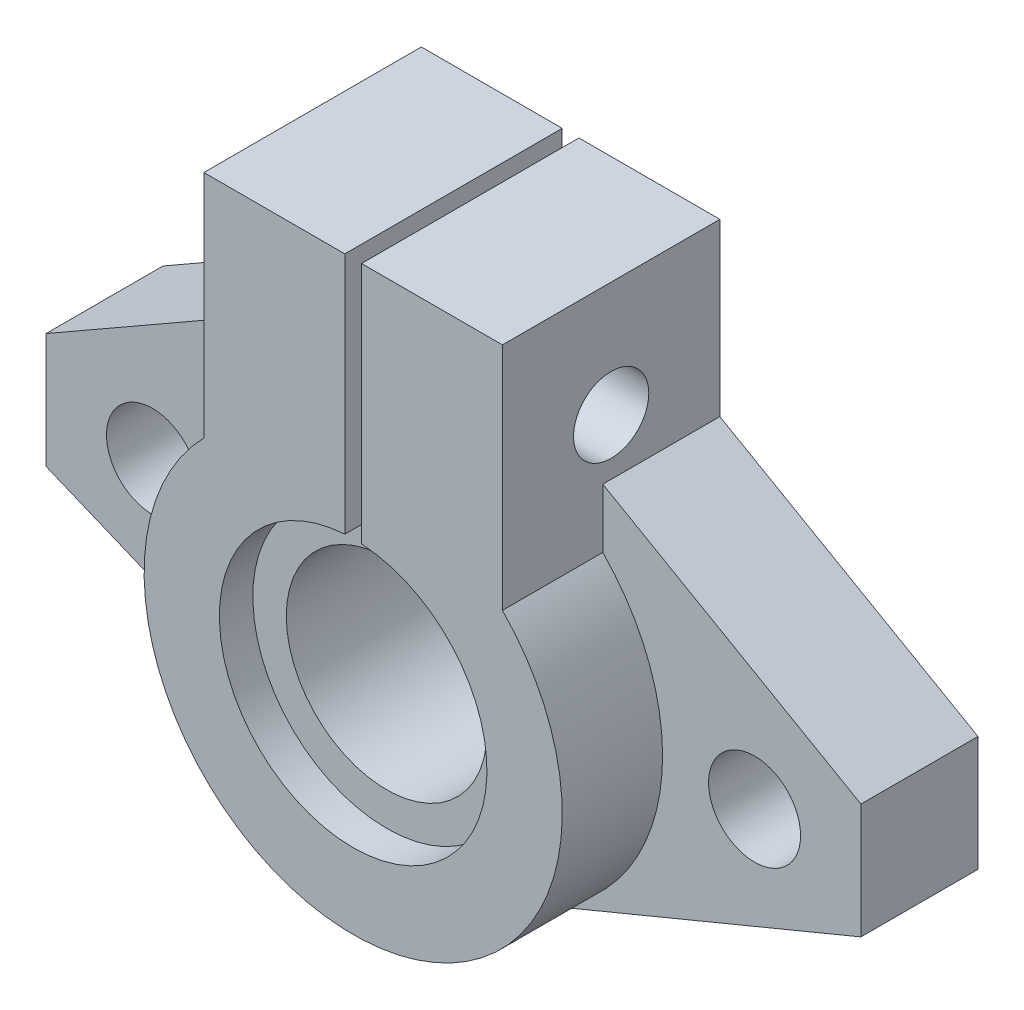
ISO-10303-21;
HEADER;
FILE_DESCRIPTION(('STEP AP214'),'2;1');
FILE_NAME('part.step','',(''),(''),'','','');
FILE_SCHEMA(('AUTOMOTIVE_DESIGN { 1 0 10303 214 1 1 1 1 }'));
ENDSEC;
DATA;
#1=APPLICATION_CONTEXT('core data for automotive mechanical design processes');
#2=APPLICATION_PROTOCOL_DEFINITION('international standard','automotive_design',2000,#1);
#3=PRODUCT_CONTEXT('',#1,'mechanical');
#4=PRODUCT('Part','Part','',(#3));
#5=PRODUCT_RELATED_PRODUCT_CATEGORY('part','',(#4));
#6=PRODUCT_DEFINITION_FORMATION('','',#4);
#7=PRODUCT_DEFINITION_CONTEXT('part definition',#1,'design');
#8=PRODUCT_DEFINITION('design','',#6,#7);
#9=PRODUCT_DEFINITION_SHAPE('','',#8);
#10=(LENGTH_UNIT() NAMED_UNIT(*) SI_UNIT(.MILLI.,.METRE.));
#11=(NAMED_UNIT(*) PLANE_ANGLE_UNIT() SI_UNIT($,.RADIAN.));
#12=(NAMED_UNIT(*) SI_UNIT($,.STERADIAN.) SOLID_ANGLE_UNIT());
#13=UNCERTAINTY_MEASURE_WITH_UNIT(LENGTH_MEASURE(1.E-05),#10,'distance_accuracy_value','');
#14=(GEOMETRIC_REPRESENTATION_CONTEXT(3) GLOBAL_UNCERTAINTY_ASSIGNED_CONTEXT((#13)) GLOBAL_UNIT_ASSIGNED_CONTEXT((#10,
#11,#12)) REPRESENTATION_CONTEXT('',''));
#15=CARTESIAN_POINT('',(0.,0.,0.));
#16=DIRECTION('',(0.,0.,1.));
#17=DIRECTION('',(1.,0.,0.));
#18=AXIS2_PLACEMENT_3D('',#15,#16,#17);
#19=CARTESIAN_POINT('',(-8.925,22.5,13.));
#20=DIRECTION('',(0.,-1.,0.));
#21=DIRECTION('',(0.,0.,-1.));
#22=AXIS2_PLACEMENT_3D('',#19,#20,#21);
#23=PLANE('',#22);
#24=DIRECTION('',(-1.,0.,0.));
#25=VECTOR('',#24,1.);
#26=CARTESIAN_POINT('',(-8.925,22.5,0.));
#27=LINE('',#26,#25);
#28=CARTESIAN_POINT('',(8.925,22.5,0.));
#29=VERTEX_POINT('',#28);
#30=CARTESIAN_POINT('',(0.5,22.5,0.));
#31=VERTEX_POINT('',#30);
#32=EDGE_CURVE('E194',#29,#31,#27,.T.);
#33=ORIENTED_EDGE('',*,*,#32,.T.);
#34=DIRECTION('',(0.,0.,1.));
#35=VECTOR('',#34,1.);
#36=CARTESIAN_POINT('',(0.5,22.5,0.));
#37=LINE('',#36,#35);
#38=CARTESIAN_POINT('',(0.5,22.5,13.));
#39=VERTEX_POINT('',#38);
#40=EDGE_CURVE('E416',#31,#39,#37,.T.);
#41=ORIENTED_EDGE('',*,*,#40,.T.);
#42=DIRECTION('',(-1.,0.,0.));
#43=VECTOR('',#42,1.);
#44=CARTESIAN_POINT('',(-8.925,22.5,13.));
#45=LINE('',#44,#43);
#46=CARTESIAN_POINT('',(8.925,22.5,13.));
#47=VERTEX_POINT('',#46);
#48=EDGE_CURVE('E201',#47,#39,#45,.T.);
#49=ORIENTED_EDGE('',*,*,#48,.F.);
#50=DIRECTION('',(0.,0.,-1.));
#51=VECTOR('',#50,1.);
#52=CARTESIAN_POINT('',(8.925,22.5,13.));
#53=LINE('',#52,#51);
#54=EDGE_CURVE('E205',#47,#29,#53,.T.);
#55=ORIENTED_EDGE('',*,*,#54,.T.);
#56=EDGE_LOOP('',(#33,#41,#49,#55));
#57=FACE_BOUND('',#56,.T.);
#58=ADVANCED_FACE('F43',(#57),#23,.F.);
#59=CARTESIAN_POINT('',(0.,0.,13.));
#60=DIRECTION('',(0.,0.,-1.));
#61=DIRECTION('',(-1.,0.,0.));
#62=AXIS2_PLACEMENT_3D('',#59,#60,#61);
#63=CYLINDRICAL_SURFACE('',#62,12.5);
#64=DIRECTION('',(0.,0.,-1.));
#65=VECTOR('',#64,1.);
#66=CARTESIAN_POINT('',(4.78354290456363,-11.5484941563911,7.));
#67=LINE('',#66,#65);
#68=CARTESIAN_POINT('',(4.78354290456363,-11.5484941563911,7.));
#69=VERTEX_POINT('',#68);
#70=CARTESIAN_POINT('',(4.78354290456363,-11.5484941563911,0.));
#71=VERTEX_POINT('',#70);
#72=EDGE_CURVE('E261',#69,#71,#67,.T.);
#73=ORIENTED_EDGE('',*,*,#72,.F.);
#74=CARTESIAN_POINT('',(0.,0.,7.));
#75=DIRECTION('',(0.,0.,1.));
#76=DIRECTION('',(1.,0.,0.));
#77=AXIS2_PLACEMENT_3D('',#74,#75,#76);
#78=CIRCLE('',#77,12.5);
#79=CARTESIAN_POINT('',(8.925,8.75182123903362,7.));
#80=VERTEX_POINT('',#79);
#81=EDGE_CURVE('E377',#69,#80,#78,.T.);
#82=ORIENTED_EDGE('',*,*,#81,.T.);
#83=DIRECTION('',(0.,0.,-1.));
#84=VECTOR('',#83,1.);
#85=CARTESIAN_POINT('',(8.925,8.75182123903362,13.));
#86=LINE('',#85,#84);
#87=CARTESIAN_POINT('',(8.925,8.75182123903362,13.));
#88=VERTEX_POINT('',#87);
#89=EDGE_CURVE('E206',#88,#80,#86,.T.);
#90=ORIENTED_EDGE('',*,*,#89,.F.);
#91=CARTESIAN_POINT('',(0.,0.,13.));
#92=DIRECTION('',(0.,0.,1.));
#93=DIRECTION('',(1.,0.,0.));
#94=AXIS2_PLACEMENT_3D('',#91,#92,#93);
#95=CIRCLE('',#94,12.5);
#96=CARTESIAN_POINT('',(-8.925,8.75182123903362,13.));
#97=VERTEX_POINT('',#96);
#98=EDGE_CURVE('E213',#97,#88,#95,.T.);
#99=ORIENTED_EDGE('',*,*,#98,.F.);
#100=DIRECTION('',(0.,0.,-1.));
#101=VECTOR('',#100,1.);
#102=CARTESIAN_POINT('',(-8.925,8.75182123903362,13.));
#103=LINE('',#102,#101);
#104=CARTESIAN_POINT('',(-8.925,8.75182123903362,7.));
#105=VERTEX_POINT('',#104);
#106=EDGE_CURVE('E207',#97,#105,#103,.T.);
#107=ORIENTED_EDGE('',*,*,#106,.T.);
#108=CARTESIAN_POINT('',(0.,0.,7.));
#109=DIRECTION('',(0.,0.,1.));
#110=DIRECTION('',(1.,0.,0.));
#111=AXIS2_PLACEMENT_3D('',#108,#109,#110);
#112=CIRCLE('',#111,12.5);
#113=CARTESIAN_POINT('',(-4.78354290456363,-11.5484941563911,7.));
#114=VERTEX_POINT('',#113);
#115=EDGE_CURVE('E277',#105,#114,#112,.T.);
#116=ORIENTED_EDGE('',*,*,#115,.T.);
#117=DIRECTION('',(0.,0.,-1.));
#118=VECTOR('',#117,1.);
#119=CARTESIAN_POINT('',(-4.78354290456363,-11.5484941563911,7.));
#120=LINE('',#119,#118);
#121=CARTESIAN_POINT('',(-4.78354290456363,-11.5484941563911,0.));
#122=VERTEX_POINT('',#121);
#123=EDGE_CURVE('E280',#114,#122,#120,.T.);
#124=ORIENTED_EDGE('',*,*,#123,.T.);
#125=CARTESIAN_POINT('',(0.,0.,0.));
#126=DIRECTION('',(0.,0.,1.));
#127=DIRECTION('',(1.,0.,0.));
#128=AXIS2_PLACEMENT_3D('',#125,#126,#127);
#129=CIRCLE('',#128,12.5);
#130=EDGE_CURVE('E215',#122,#71,#129,.T.);
#131=ORIENTED_EDGE('',*,*,#130,.T.);
#132=EDGE_LOOP('',(#73,#82,#90,#99,#107,#116,#124,#131));
#133=FACE_BOUND('',#132,.T.);
#134=ADVANCED_FACE('F44',(#133),#63,.T.);
#135=CARTESIAN_POINT('',(8.925,22.5,13.));
#136=DIRECTION('',(-1.,0.,0.));
#137=DIRECTION('',(0.,0.,1.));
#138=AXIS2_PLACEMENT_3D('',#135,#136,#137);
#139=PLANE('',#138);
#140=CARTESIAN_POINT('',(8.925,15.6259106195168,6.5));
#141=DIRECTION('',(1.,0.,0.));
#142=DIRECTION('',(0.,0.,-1.));
#143=AXIS2_PLACEMENT_3D('',#140,#141,#142);
#144=CIRCLE('',#143,2.25);
#145=CARTESIAN_POINT('',(8.925,15.6259106195168,4.25));
#146=VERTEX_POINT('',#145);
#147=EDGE_CURVE('E436',#146,#146,#144,.T.);
#148=ORIENTED_EDGE('',*,*,#147,.F.);
#149=EDGE_LOOP('',(#148));
#150=FACE_BOUND('',#149,.T.);
#151=DIRECTION('',(0.,0.,-1.));
#152=VECTOR('',#151,1.);
#153=CARTESIAN_POINT('',(8.925,12.2859520739162,7.));
#154=LINE('',#153,#152);
#155=CARTESIAN_POINT('',(8.925,12.2859520739162,7.));
#156=VERTEX_POINT('',#155);
#157=CARTESIAN_POINT('',(8.925,12.2859520739162,0.));
#158=VERTEX_POINT('',#157);
#159=EDGE_CURVE('E402',#156,#158,#154,.T.);
#160=ORIENTED_EDGE('',*,*,#159,.T.);
#161=DIRECTION('',(0.,1.,0.));
#162=VECTOR('',#161,1.);
#163=CARTESIAN_POINT('',(8.925,22.5,0.));
#164=LINE('',#163,#162);
#165=EDGE_CURVE('E195',#158,#29,#164,.T.);
#166=ORIENTED_EDGE('',*,*,#165,.T.);
#167=ORIENTED_EDGE('',*,*,#54,.F.);
#168=DIRECTION('',(0.,1.,0.));
#169=VECTOR('',#168,1.);
#170=CARTESIAN_POINT('',(8.925,22.5,13.));
#171=LINE('',#170,#169);
#172=EDGE_CURVE('E243',#88,#47,#171,.T.);
#173=ORIENTED_EDGE('',*,*,#172,.F.);
#174=ORIENTED_EDGE('',*,*,#89,.T.);
#175=DIRECTION('',(0.,-1.,0.));
#176=VECTOR('',#175,1.);
#177=CARTESIAN_POINT('',(8.925,0.,7.));
#178=LINE('',#177,#176);
#179=EDGE_CURVE('E384',#156,#80,#178,.T.);
#180=ORIENTED_EDGE('',*,*,#179,.F.);
#181=EDGE_LOOP('',(#160,#166,#167,#173,#174,#180));
#182=FACE_BOUND('',#181,.T.);
#183=ADVANCED_FACE('F324',(#150,#182),#139,.F.);
#184=CARTESIAN_POINT('',(0.,0.,0.));
#185=DIRECTION('',(0.,0.,1.));
#186=DIRECTION('',(1.,0.,0.));
#187=AXIS2_PLACEMENT_3D('',#184,#185,#186);
#188=CYLINDRICAL_SURFACE('',#187,6.);
#189=CARTESIAN_POINT('',(0.,0.,11.));
#190=DIRECTION('',(0.,0.,1.));
#191=DIRECTION('',(1.,0.,0.));
#192=AXIS2_PLACEMENT_3D('',#189,#190,#191);
#193=CIRCLE('',#192,6.);
#194=CARTESIAN_POINT('',(0.5,5.9791303715507,11.));
#195=VERTEX_POINT('',#194);
#196=CARTESIAN_POINT('',(-0.5,5.9791303715507,11.));
#197=VERTEX_POINT('',#196);
#198=EDGE_CURVE('E220',#195,#197,#193,.F.);
#199=ORIENTED_EDGE('',*,*,#198,.F.);
#200=DIRECTION('',(0.,0.,1.));
#201=VECTOR('',#200,1.);
#202=CARTESIAN_POINT('',(0.5,5.9791303715507,0.));
#203=LINE('',#202,#201);
#204=CARTESIAN_POINT('',(0.5,5.9791303715507,0.));
#205=VERTEX_POINT('',#204);
#206=EDGE_CURVE('E423',#205,#195,#203,.T.);
#207=ORIENTED_EDGE('',*,*,#206,.F.);
#208=CARTESIAN_POINT('',(0.,0.,0.));
#209=DIRECTION('',(0.,0.,1.));
#210=DIRECTION('',(1.,0.,0.));
#211=AXIS2_PLACEMENT_3D('',#208,#209,#210);
#212=CIRCLE('',#211,6.);
#213=CARTESIAN_POINT('',(-0.5,5.9791303715507,0.));
#214=VERTEX_POINT('',#213);
#215=EDGE_CURVE('E219',#214,#205,#212,.T.);
#216=ORIENTED_EDGE('',*,*,#215,.F.);
#217=DIRECTION('',(0.,0.,1.));
#218=VECTOR('',#217,1.);
#219=CARTESIAN_POINT('',(-0.5,5.9791303715507,0.));
#220=LINE('',#219,#218);
#221=EDGE_CURVE('E171',#214,#197,#220,.T.);
#222=ORIENTED_EDGE('',*,*,#221,.T.);
#223=EDGE_LOOP('',(#199,#207,#216,#222));
#224=FACE_BOUND('',#223,.T.);
#225=ADVANCED_FACE('F350',(#224),#188,.F.);
#226=CARTESIAN_POINT('',(0.,0.,13.));
#227=DIRECTION('',(0.,0.,1.));
#228=DIRECTION('',(1.,0.,0.));
#229=AXIS2_PLACEMENT_3D('',#226,#227,#228);
#230=PLANE('',#229);
#231=DIRECTION('',(0.,1.,0.));
#232=VECTOR('',#231,1.);
#233=CARTESIAN_POINT('',(0.5,5.9791303715507,13.));
#234=LINE('',#233,#232);
#235=CARTESIAN_POINT('',(0.5,7.98435971133565,13.));
#236=VERTEX_POINT('',#235);
#237=EDGE_CURVE('E179',#236,#39,#234,.T.);
#238=ORIENTED_EDGE('',*,*,#237,.F.);
#239=CARTESIAN_POINT('',(0.,0.,13.));
#240=DIRECTION('',(0.,0.,1.));
#241=DIRECTION('',(1.,0.,0.));
#242=AXIS2_PLACEMENT_3D('',#239,#240,#241);
#243=CIRCLE('',#242,8.);
#244=CARTESIAN_POINT('',(-0.5,7.98435971133565,13.));
#245=VERTEX_POINT('',#244);
#246=EDGE_CURVE('E227',#245,#236,#243,.T.);
#247=ORIENTED_EDGE('',*,*,#246,.F.);
#248=DIRECTION('',(0.,-1.,0.));
#249=VECTOR('',#248,1.);
#250=CARTESIAN_POINT('',(-0.5,5.9791303715507,13.));
#251=LINE('',#250,#249);
#252=CARTESIAN_POINT('',(-0.5,22.5,13.));
#253=VERTEX_POINT('',#252);
#254=EDGE_CURVE('E56',#253,#245,#251,.T.);
#255=ORIENTED_EDGE('',*,*,#254,.F.);
#256=CARTESIAN_POINT('',(-8.925,22.5,13.));
#257=VERTEX_POINT('',#256);
#258=EDGE_CURVE('E183',#253,#257,#45,.T.);
#259=ORIENTED_EDGE('',*,*,#258,.T.);
#260=DIRECTION('',(0.,-1.,0.));
#261=VECTOR('',#260,1.);
#262=CARTESIAN_POINT('',(-8.925,22.5,13.));
#263=LINE('',#262,#261);
#264=EDGE_CURVE('E198',#257,#97,#263,.T.);
#265=ORIENTED_EDGE('',*,*,#264,.T.);
#266=ORIENTED_EDGE('',*,*,#98,.T.);
#267=ORIENTED_EDGE('',*,*,#172,.T.);
#268=ORIENTED_EDGE('',*,*,#48,.T.);
#269=EDGE_LOOP('',(#238,#247,#255,#259,#265,#266,#267,#268));
#270=FACE_BOUND('',#269,.T.);
#271=ADVANCED_FACE('F234',(#270),#230,.T.);
#272=CARTESIAN_POINT('',(0.,0.,0.));
#273=DIRECTION('',(0.,0.,1.));
#274=DIRECTION('',(1.,0.,0.));
#275=AXIS2_PLACEMENT_3D('',#272,#273,#274);
#276=PLANE('',#275);
#277=ORIENTED_EDGE('',*,*,#215,.T.);
#278=DIRECTION('',(0.,1.,0.));
#279=VECTOR('',#278,1.);
#280=CARTESIAN_POINT('',(0.5,5.9791303715507,0.));
#281=LINE('',#280,#279);
#282=EDGE_CURVE('E177',#205,#31,#281,.T.);
#283=ORIENTED_EDGE('',*,*,#282,.T.);
#284=ORIENTED_EDGE('',*,*,#32,.F.);
#285=ORIENTED_EDGE('',*,*,#165,.F.);
#286=DIRECTION('',(-0.867602640598347,0.497258140231787,0.));
#287=VECTOR('',#286,1.);
#288=CARTESIAN_POINT('',(7.5072818557886,13.0985036439266,0.));
#289=LINE('',#288,#287);
#290=CARTESIAN_POINT('',(24.3591794673459,3.44,0.));
#291=VERTEX_POINT('',#290);
#292=EDGE_CURVE('E386',#291,#158,#289,.T.);
#293=ORIENTED_EDGE('',*,*,#292,.F.);
#294=DIRECTION('',(0.,-1.,0.));
#295=VECTOR('',#294,1.);
#296=CARTESIAN_POINT('',(24.3591794673459,0.,0.));
#297=LINE('',#296,#295);
#298=CARTESIAN_POINT('',(24.3591794673459,-3.44,0.));
#299=VERTEX_POINT('',#298);
#300=EDGE_CURVE('E401',#291,#299,#297,.T.);
#301=ORIENTED_EDGE('',*,*,#300,.T.);
#302=DIRECTION('',(0.923879532511287,0.38268343236509,0.));
#303=VECTOR('',#302,1.);
#304=CARTESIAN_POINT('',(4.78354290456363,-11.5484941563911,0.));
#305=LINE('',#304,#303);
#306=EDGE_CURVE('E367',#71,#299,#305,.T.);
#307=ORIENTED_EDGE('',*,*,#306,.F.);
#308=ORIENTED_EDGE('',*,*,#130,.F.);
#309=DIRECTION('',(-0.923879532511287,0.38268343236509,0.));
#310=VECTOR('',#309,1.);
#311=CARTESIAN_POINT('',(-4.78354290456363,-11.5484941563911,0.));
#312=LINE('',#311,#310);
#313=CARTESIAN_POINT('',(-24.3661310458058,-3.43712056192201,0.));
#314=VERTEX_POINT('',#313);
#315=EDGE_CURVE('E263',#122,#314,#312,.T.);
#316=ORIENTED_EDGE('',*,*,#315,.T.);
#317=DIRECTION('',(0.,-1.,0.));
#318=VECTOR('',#317,1.);
#319=CARTESIAN_POINT('',(-24.3661310458058,0.,0.));
#320=LINE('',#319,#318);
#321=CARTESIAN_POINT('',(-24.3661310458058,3.44,0.));
#322=VERTEX_POINT('',#321);
#323=EDGE_CURVE('E257',#322,#314,#320,.T.);
#324=ORIENTED_EDGE('',*,*,#323,.F.);
#325=DIRECTION('',(0.86769921537807,0.497089601211171,0.));
#326=VECTOR('',#325,1.);
#327=CARTESIAN_POINT('',(-7.50457943844383,13.0996860015059,0.));
#328=LINE('',#327,#326);
#329=CARTESIAN_POINT('',(-8.925,12.2859520739162,0.));
#330=VERTEX_POINT('',#329);
#331=EDGE_CURVE('E255',#322,#330,#328,.T.);
#332=ORIENTED_EDGE('',*,*,#331,.T.);
#333=DIRECTION('',(0.,-1.,0.));
#334=VECTOR('',#333,1.);
#335=CARTESIAN_POINT('',(-8.925,22.5,0.));
#336=LINE('',#335,#334);
#337=CARTESIAN_POINT('',(-8.925,22.5,0.));
#338=VERTEX_POINT('',#337);
#339=EDGE_CURVE('E192',#338,#330,#336,.T.);
#340=ORIENTED_EDGE('',*,*,#339,.F.);
#341=CARTESIAN_POINT('',(-0.5,22.5,0.));
#342=VERTEX_POINT('',#341);
#343=EDGE_CURVE('E181',#342,#338,#27,.T.);
#344=ORIENTED_EDGE('',*,*,#343,.F.);
#345=DIRECTION('',(0.,-1.,0.));
#346=VECTOR('',#345,1.);
#347=CARTESIAN_POINT('',(-0.5,5.9791303715507,0.));
#348=LINE('',#347,#346);
#349=EDGE_CURVE('E167',#342,#214,#348,.T.);
#350=ORIENTED_EDGE('',*,*,#349,.T.);
#351=EDGE_LOOP('',(#277,#283,#284,#285,#293,#301,#307,#308,#316,#324,#332,#340,#344,#350));
#352=FACE_BOUND('',#351,.T.);
#353=CARTESIAN_POINT('',(-18.,0.,0.));
#354=DIRECTION('',(0.,0.,1.));
#355=DIRECTION('',(1.,0.,0.));
#356=AXIS2_PLACEMENT_3D('',#353,#354,#355);
#357=CIRCLE('',#356,2.75);
#358=CARTESIAN_POINT('',(-15.25,0.,0.));
#359=VERTEX_POINT('',#358);
#360=EDGE_CURVE('E272',#359,#359,#357,.T.);
#361=ORIENTED_EDGE('',*,*,#360,.T.);
#362=EDGE_LOOP('',(#361));
#363=FACE_BOUND('',#362,.T.);
#364=CARTESIAN_POINT('',(18.,0.,0.));
#365=DIRECTION('',(0.,0.,1.));
#366=DIRECTION('',(1.,0.,0.));
#367=AXIS2_PLACEMENT_3D('',#364,#365,#366);
#368=CIRCLE('',#367,2.75);
#369=CARTESIAN_POINT('',(20.75,0.,0.));
#370=VERTEX_POINT('',#369);
#371=EDGE_CURVE('E387',#370,#370,#368,.T.);
#372=ORIENTED_EDGE('',*,*,#371,.T.);
#373=EDGE_LOOP('',(#372));
#374=FACE_BOUND('',#373,.T.);
#375=ADVANCED_FACE('F189',(#352,#363,#374),#276,.F.);
#376=CARTESIAN_POINT('',(-8.925,22.5,13.));
#377=DIRECTION('',(1.,0.,0.));
#378=DIRECTION('',(0.,0.,-1.));
#379=AXIS2_PLACEMENT_3D('',#376,#377,#378);
#380=PLANE('',#379);
#381=CARTESIAN_POINT('',(-8.925,15.6259106195168,6.5));
#382=DIRECTION('',(1.,0.,0.));
#383=DIRECTION('',(0.,0.,-1.));
#384=AXIS2_PLACEMENT_3D('',#381,#382,#383);
#385=CIRCLE('',#384,2.25);
#386=CARTESIAN_POINT('',(-8.925,15.6259106195168,4.25));
#387=VERTEX_POINT('',#386);
#388=EDGE_CURVE('E429',#387,#387,#385,.T.);
#389=ORIENTED_EDGE('',*,*,#388,.T.);
#390=EDGE_LOOP('',(#389));
#391=FACE_BOUND('',#390,.T.);
#392=ORIENTED_EDGE('',*,*,#339,.T.);
#393=DIRECTION('',(0.,0.,-1.));
#394=VECTOR('',#393,1.);
#395=CARTESIAN_POINT('',(-8.925,12.2859520739162,7.));
#396=LINE('',#395,#394);
#397=CARTESIAN_POINT('',(-8.925,12.2859520739162,7.));
#398=VERTEX_POINT('',#397);
#399=EDGE_CURVE('E231',#398,#330,#396,.T.);
#400=ORIENTED_EDGE('',*,*,#399,.F.);
#401=DIRECTION('',(0.,-1.,0.));
#402=VECTOR('',#401,1.);
#403=CARTESIAN_POINT('',(-8.925,0.,7.));
#404=LINE('',#403,#402);
#405=EDGE_CURVE('E294',#398,#105,#404,.T.);
#406=ORIENTED_EDGE('',*,*,#405,.T.);
#407=ORIENTED_EDGE('',*,*,#106,.F.);
#408=ORIENTED_EDGE('',*,*,#264,.F.);
#409=DIRECTION('',(0.,0.,-1.));
#410=VECTOR('',#409,1.);
#411=CARTESIAN_POINT('',(-8.925,22.5,13.));
#412=LINE('',#411,#410);
#413=EDGE_CURVE('E199',#257,#338,#412,.T.);
#414=ORIENTED_EDGE('',*,*,#413,.T.);
#415=EDGE_LOOP('',(#392,#400,#406,#407,#408,#414));
#416=FACE_BOUND('',#415,.T.);
#417=ADVANCED_FACE('F249',(#391,#416),#380,.F.);
#418=ORIENTED_EDGE('',*,*,#258,.F.);
#419=DIRECTION('',(0.,0.,1.));
#420=VECTOR('',#419,1.);
#421=CARTESIAN_POINT('',(-0.5,22.5,0.));
#422=LINE('',#421,#420);
#423=EDGE_CURVE('E166',#342,#253,#422,.T.);
#424=ORIENTED_EDGE('',*,*,#423,.F.);
#425=ORIENTED_EDGE('',*,*,#343,.T.);
#426=ORIENTED_EDGE('',*,*,#413,.F.);
#427=EDGE_LOOP('',(#418,#424,#425,#426));
#428=FACE_BOUND('',#427,.T.);
#429=ADVANCED_FACE('F182',(#428),#23,.F.);
#430=CARTESIAN_POINT('',(0.,0.,11.));
#431=DIRECTION('',(0.,0.,1.));
#432=DIRECTION('',(1.,0.,0.));
#433=AXIS2_PLACEMENT_3D('',#430,#431,#432);
#434=PLANE('',#433);
#435=DIRECTION('',(0.,1.,0.));
#436=VECTOR('',#435,1.);
#437=CARTESIAN_POINT('',(0.5,0.,11.));
#438=LINE('',#437,#436);
#439=CARTESIAN_POINT('',(0.5,7.98435971133565,11.));
#440=VERTEX_POINT('',#439);
#441=EDGE_CURVE('E69',#195,#440,#438,.T.);
#442=ORIENTED_EDGE('',*,*,#441,.F.);
#443=ORIENTED_EDGE('',*,*,#198,.T.);
#444=DIRECTION('',(0.,-1.,0.));
#445=VECTOR('',#444,1.);
#446=CARTESIAN_POINT('',(-0.5,0.,11.));
#447=LINE('',#446,#445);
#448=CARTESIAN_POINT('',(-0.5,7.98435971133565,11.));
#449=VERTEX_POINT('',#448);
#450=EDGE_CURVE('E419',#449,#197,#447,.T.);
#451=ORIENTED_EDGE('',*,*,#450,.F.);
#452=CARTESIAN_POINT('',(0.,0.,11.));
#453=DIRECTION('',(0.,0.,1.));
#454=DIRECTION('',(1.,0.,0.));
#455=AXIS2_PLACEMENT_3D('',#452,#453,#454);
#456=CIRCLE('',#455,8.);
#457=EDGE_CURVE('E222',#449,#440,#456,.T.);
#458=ORIENTED_EDGE('',*,*,#457,.T.);
#459=EDGE_LOOP('',(#442,#443,#451,#458));
#460=FACE_BOUND('',#459,.T.);
#461=ADVANCED_FACE('F329',(#460),#434,.T.);
#462=CARTESIAN_POINT('',(0.,0.,11.));
#463=DIRECTION('',(0.,0.,1.));
#464=DIRECTION('',(1.,0.,0.));
#465=AXIS2_PLACEMENT_3D('',#462,#463,#464);
#466=CYLINDRICAL_SURFACE('',#465,8.);
#467=ORIENTED_EDGE('',*,*,#246,.T.);
#468=DIRECTION('',(0.,0.,1.));
#469=VECTOR('',#468,1.);
#470=CARTESIAN_POINT('',(0.5,7.98435971133565,11.));
#471=LINE('',#470,#469);
#472=EDGE_CURVE('E11',#236,#440,#471,.F.);
#473=ORIENTED_EDGE('',*,*,#472,.T.);
#474=ORIENTED_EDGE('',*,*,#457,.F.);
#475=DIRECTION('',(0.,0.,1.));
#476=VECTOR('',#475,1.);
#477=CARTESIAN_POINT('',(-0.5,7.98435971133565,11.));
#478=LINE('',#477,#476);
#479=EDGE_CURVE('E55',#449,#245,#478,.T.);
#480=ORIENTED_EDGE('',*,*,#479,.T.);
#481=EDGE_LOOP('',(#467,#473,#474,#480));
#482=FACE_BOUND('',#481,.T.);
#483=ADVANCED_FACE('F226',(#482),#466,.F.);
#484=CARTESIAN_POINT('',(-7.50457943844383,13.0996860015059,7.));
#485=DIRECTION('',(-0.497089601211171,0.86769921537807,0.));
#486=DIRECTION('',(-0.86769921537807,-0.497089601211171,0.));
#487=AXIS2_PLACEMENT_3D('',#484,#485,#486);
#488=PLANE('',#487);
#489=ORIENTED_EDGE('',*,*,#331,.F.);
#490=DIRECTION('',(0.,0.,-1.));
#491=VECTOR('',#490,1.);
#492=CARTESIAN_POINT('',(-24.3661310458058,3.44,7.));
#493=LINE('',#492,#491);
#494=CARTESIAN_POINT('',(-24.3661310458058,3.44,7.));
#495=VERTEX_POINT('',#494);
#496=EDGE_CURVE('E236',#495,#322,#493,.T.);
#497=ORIENTED_EDGE('',*,*,#496,.F.);
#498=DIRECTION('',(0.86769921537807,0.497089601211171,0.));
#499=VECTOR('',#498,1.);
#500=CARTESIAN_POINT('',(-7.50457943844383,13.0996860015059,7.));
#501=LINE('',#500,#499);
#502=EDGE_CURVE('E258',#495,#398,#501,.T.);
#503=ORIENTED_EDGE('',*,*,#502,.T.);
#504=ORIENTED_EDGE('',*,*,#399,.T.);
#505=EDGE_LOOP('',(#489,#497,#503,#504));
#506=FACE_BOUND('',#505,.T.);
#507=ADVANCED_FACE('F251',(#506),#488,.T.);
#508=CARTESIAN_POINT('',(-24.3661310458058,0.,7.));
#509=DIRECTION('',(1.,0.,0.));
#510=DIRECTION('',(0.,0.,-1.));
#511=AXIS2_PLACEMENT_3D('',#508,#509,#510);
#512=PLANE('',#511);
#513=ORIENTED_EDGE('',*,*,#323,.T.);
#514=DIRECTION('',(0.,0.,-1.));
#515=VECTOR('',#514,1.);
#516=CARTESIAN_POINT('',(-24.3661310458058,-3.43712056192201,7.));
#517=LINE('',#516,#515);
#518=CARTESIAN_POINT('',(-24.3661310458058,-3.43712056192201,7.));
#519=VERTEX_POINT('',#518);
#520=EDGE_CURVE('E276',#519,#314,#517,.T.);
#521=ORIENTED_EDGE('',*,*,#520,.F.);
#522=DIRECTION('',(0.,-1.,0.));
#523=VECTOR('',#522,1.);
#524=CARTESIAN_POINT('',(-24.3661310458058,0.,7.));
#525=LINE('',#524,#523);
#526=EDGE_CURVE('E285',#495,#519,#525,.T.);
#527=ORIENTED_EDGE('',*,*,#526,.F.);
#528=ORIENTED_EDGE('',*,*,#496,.T.);
#529=EDGE_LOOP('',(#513,#521,#527,#528));
#530=FACE_BOUND('',#529,.T.);
#531=ADVANCED_FACE('F284',(#530),#512,.F.);
#532=CARTESIAN_POINT('',(-4.78354290456363,-11.5484941563911,7.));
#533=DIRECTION('',(-0.38268343236509,-0.923879532511287,0.));
#534=DIRECTION('',(0.923879532511287,-0.38268343236509,0.));
#535=AXIS2_PLACEMENT_3D('',#532,#533,#534);
#536=PLANE('',#535);
#537=ORIENTED_EDGE('',*,*,#315,.F.);
#538=ORIENTED_EDGE('',*,*,#123,.F.);
#539=DIRECTION('',(-0.923879532511287,0.38268343236509,0.));
#540=VECTOR('',#539,1.);
#541=CARTESIAN_POINT('',(-4.78354290456363,-11.5484941563911,7.));
#542=LINE('',#541,#540);
#543=EDGE_CURVE('E286',#114,#519,#542,.T.);
#544=ORIENTED_EDGE('',*,*,#543,.T.);
#545=ORIENTED_EDGE('',*,*,#520,.T.);
#546=EDGE_LOOP('',(#537,#538,#544,#545));
#547=FACE_BOUND('',#546,.T.);
#548=ADVANCED_FACE('F312',(#547),#536,.T.);
#549=CARTESIAN_POINT('',(-18.,0.,7.));
#550=DIRECTION('',(0.,0.,-1.));
#551=DIRECTION('',(-1.,0.,0.));
#552=AXIS2_PLACEMENT_3D('',#549,#550,#551);
#553=CYLINDRICAL_SURFACE('',#552,2.75);
#554=CARTESIAN_POINT('',(-18.,0.,7.));
#555=DIRECTION('',(0.,0.,1.));
#556=DIRECTION('',(1.,0.,0.));
#557=AXIS2_PLACEMENT_3D('',#554,#555,#556);
#558=CIRCLE('',#557,2.75);
#559=CARTESIAN_POINT('',(-15.25,0.,7.));
#560=VERTEX_POINT('',#559);
#561=EDGE_CURVE('E267',#560,#560,#558,.T.);
#562=ORIENTED_EDGE('',*,*,#561,.T.);
#563=EDGE_LOOP('',(#562));
#564=FACE_BOUND('',#563,.T.);
#565=ORIENTED_EDGE('',*,*,#360,.F.);
#566=EDGE_LOOP('',(#565));
#567=FACE_BOUND('',#566,.T.);
#568=ADVANCED_FACE('F305',(#564,#567),#553,.F.);
#569=CARTESIAN_POINT('',(0.,0.,7.));
#570=DIRECTION('',(0.,0.,1.));
#571=DIRECTION('',(1.,0.,0.));
#572=AXIS2_PLACEMENT_3D('',#569,#570,#571);
#573=PLANE('',#572);
#574=ORIENTED_EDGE('',*,*,#115,.F.);
#575=ORIENTED_EDGE('',*,*,#405,.F.);
#576=ORIENTED_EDGE('',*,*,#502,.F.);
#577=ORIENTED_EDGE('',*,*,#526,.T.);
#578=ORIENTED_EDGE('',*,*,#543,.F.);
#579=EDGE_LOOP('',(#574,#575,#576,#577,#578));
#580=FACE_BOUND('',#579,.T.);
#581=ORIENTED_EDGE('',*,*,#561,.F.);
#582=EDGE_LOOP('',(#581));
#583=FACE_BOUND('',#582,.T.);
#584=ADVANCED_FACE('F295',(#580,#583),#573,.T.);
#585=CARTESIAN_POINT('',(4.78354290456363,-11.5484941563911,7.));
#586=DIRECTION('',(-0.38268343236509,0.923879532511287,0.));
#587=DIRECTION('',(-0.923879532511287,-0.38268343236509,0.));
#588=AXIS2_PLACEMENT_3D('',#585,#586,#587);
#589=PLANE('',#588);
#590=ORIENTED_EDGE('',*,*,#306,.T.);
#591=DIRECTION('',(0.,0.,-1.));
#592=VECTOR('',#591,1.);
#593=CARTESIAN_POINT('',(24.3591794673459,-3.44,7.));
#594=LINE('',#593,#592);
#595=CARTESIAN_POINT('',(24.3591794673459,-3.44,7.));
#596=VERTEX_POINT('',#595);
#597=EDGE_CURVE('E266',#596,#299,#594,.T.);
#598=ORIENTED_EDGE('',*,*,#597,.F.);
#599=DIRECTION('',(0.923879532511287,0.38268343236509,0.));
#600=VECTOR('',#599,1.);
#601=CARTESIAN_POINT('',(4.78354290456363,-11.5484941563911,7.));
#602=LINE('',#601,#600);
#603=EDGE_CURVE('E373',#69,#596,#602,.T.);
#604=ORIENTED_EDGE('',*,*,#603,.F.);
#605=ORIENTED_EDGE('',*,*,#72,.T.);
#606=EDGE_LOOP('',(#590,#598,#604,#605));
#607=FACE_BOUND('',#606,.T.);
#608=ADVANCED_FACE('F308',(#607),#589,.F.);
#609=CARTESIAN_POINT('',(24.3591794673459,0.,7.));
#610=DIRECTION('',(1.,0.,0.));
#611=DIRECTION('',(0.,0.,-1.));
#612=AXIS2_PLACEMENT_3D('',#609,#610,#611);
#613=PLANE('',#612);
#614=ORIENTED_EDGE('',*,*,#300,.F.);
#615=DIRECTION('',(0.,0.,-1.));
#616=VECTOR('',#615,1.);
#617=CARTESIAN_POINT('',(24.3591794673459,3.44,7.));
#618=LINE('',#617,#616);
#619=CARTESIAN_POINT('',(24.3591794673459,3.44,7.));
#620=VERTEX_POINT('',#619);
#621=EDGE_CURVE('E408',#620,#291,#618,.T.);
#622=ORIENTED_EDGE('',*,*,#621,.F.);
#623=DIRECTION('',(0.,-1.,0.));
#624=VECTOR('',#623,1.);
#625=CARTESIAN_POINT('',(24.3591794673459,0.,7.));
#626=LINE('',#625,#624);
#627=EDGE_CURVE('E378',#620,#596,#626,.T.);
#628=ORIENTED_EDGE('',*,*,#627,.T.);
#629=ORIENTED_EDGE('',*,*,#597,.T.);
#630=EDGE_LOOP('',(#614,#622,#628,#629));
#631=FACE_BOUND('',#630,.T.);
#632=ADVANCED_FACE('F315',(#631),#613,.T.);
#633=CARTESIAN_POINT('',(7.5072818557886,13.0985036439266,7.));
#634=DIRECTION('',(-0.497258140231787,-0.867602640598347,0.));
#635=DIRECTION('',(0.867602640598347,-0.497258140231787,0.));
#636=AXIS2_PLACEMENT_3D('',#633,#634,#635);
#637=PLANE('',#636);
#638=ORIENTED_EDGE('',*,*,#292,.T.);
#639=ORIENTED_EDGE('',*,*,#159,.F.);
#640=DIRECTION('',(-0.867602640598347,0.497258140231787,0.));
#641=VECTOR('',#640,1.);
#642=CARTESIAN_POINT('',(7.5072818557886,13.0985036439266,7.));
#643=LINE('',#642,#641);
#644=EDGE_CURVE('E395',#620,#156,#643,.T.);
#645=ORIENTED_EDGE('',*,*,#644,.F.);
#646=ORIENTED_EDGE('',*,*,#621,.T.);
#647=EDGE_LOOP('',(#638,#639,#645,#646));
#648=FACE_BOUND('',#647,.T.);
#649=ADVANCED_FACE('F462',(#648),#637,.F.);
#650=CARTESIAN_POINT('',(18.,0.,7.));
#651=DIRECTION('',(0.,0.,-1.));
#652=DIRECTION('',(-1.,0.,0.));
#653=AXIS2_PLACEMENT_3D('',#650,#651,#652);
#654=CYLINDRICAL_SURFACE('',#653,2.75);
#655=CARTESIAN_POINT('',(18.,0.,7.));
#656=DIRECTION('',(0.,0.,1.));
#657=DIRECTION('',(1.,0.,0.));
#658=AXIS2_PLACEMENT_3D('',#655,#656,#657);
#659=CIRCLE('',#658,2.75);
#660=CARTESIAN_POINT('',(20.75,0.,7.));
#661=VERTEX_POINT('',#660);
#662=EDGE_CURVE('E400',#661,#661,#659,.T.);
#663=ORIENTED_EDGE('',*,*,#662,.T.);
#664=EDGE_LOOP('',(#663));
#665=FACE_BOUND('',#664,.T.);
#666=ORIENTED_EDGE('',*,*,#371,.F.);
#667=EDGE_LOOP('',(#666));
#668=FACE_BOUND('',#667,.T.);
#669=ADVANCED_FACE('F459',(#665,#668),#654,.F.);
#670=CARTESIAN_POINT('',(0.,0.,7.));
#671=DIRECTION('',(0.,0.,1.));
#672=DIRECTION('',(1.,0.,0.));
#673=AXIS2_PLACEMENT_3D('',#670,#671,#672);
#674=PLANE('',#673);
#675=ORIENTED_EDGE('',*,*,#81,.F.);
#676=ORIENTED_EDGE('',*,*,#603,.T.);
#677=ORIENTED_EDGE('',*,*,#627,.F.);
#678=ORIENTED_EDGE('',*,*,#644,.T.);
#679=ORIENTED_EDGE('',*,*,#179,.T.);
#680=EDGE_LOOP('',(#675,#676,#677,#678,#679));
#681=FACE_BOUND('',#680,.T.);
#682=ORIENTED_EDGE('',*,*,#662,.F.);
#683=EDGE_LOOP('',(#682));
#684=FACE_BOUND('',#683,.T.);
#685=ADVANCED_FACE('F385',(#681,#684),#674,.T.);
#686=CARTESIAN_POINT('',(-0.5,5.9791303715507,0.));
#687=DIRECTION('',(-1.,0.,0.));
#688=DIRECTION('',(0.,-1.,0.));
#689=AXIS2_PLACEMENT_3D('',#686,#687,#688);
#690=PLANE('',#689);
#691=CARTESIAN_POINT('',(-0.5,15.6259106195168,6.5));
#692=DIRECTION('',(-1.,0.,0.));
#693=DIRECTION('',(0.,-1.,0.));
#694=AXIS2_PLACEMENT_3D('',#691,#692,#693);
#695=CIRCLE('',#694,2.25);
#696=CARTESIAN_POINT('',(-0.5,15.6259106195168,4.25));
#697=VERTEX_POINT('',#696);
#698=EDGE_CURVE('E431',#697,#697,#695,.T.);
#699=ORIENTED_EDGE('',*,*,#698,.T.);
#700=EDGE_LOOP('',(#699));
#701=FACE_BOUND('',#700,.T.);
#702=ORIENTED_EDGE('',*,*,#450,.T.);
#703=ORIENTED_EDGE('',*,*,#221,.F.);
#704=ORIENTED_EDGE('',*,*,#349,.F.);
#705=ORIENTED_EDGE('',*,*,#423,.T.);
#706=ORIENTED_EDGE('',*,*,#254,.T.);
#707=ORIENTED_EDGE('',*,*,#479,.F.);
#708=EDGE_LOOP('',(#702,#703,#704,#705,#706,#707));
#709=FACE_BOUND('',#708,.T.);
#710=ADVANCED_FACE('F169',(#701,#709),#690,.F.);
#711=CARTESIAN_POINT('',(0.5,5.9791303715507,0.));
#712=DIRECTION('',(1.,0.,0.));
#713=DIRECTION('',(0.,1.,0.));
#714=AXIS2_PLACEMENT_3D('',#711,#712,#713);
#715=PLANE('',#714);
#716=CARTESIAN_POINT('',(0.5,15.6259106195168,6.5));
#717=DIRECTION('',(1.,0.,0.));
#718=DIRECTION('',(0.,1.,0.));
#719=AXIS2_PLACEMENT_3D('',#716,#717,#718);
#720=CIRCLE('',#719,2.25);
#721=CARTESIAN_POINT('',(0.5,17.8759106195168,6.5));
#722=VERTEX_POINT('',#721);
#723=EDGE_CURVE('E50',#722,#722,#720,.T.);
#724=ORIENTED_EDGE('',*,*,#723,.T.);
#725=EDGE_LOOP('',(#724));
#726=FACE_BOUND('',#725,.T.);
#727=ORIENTED_EDGE('',*,*,#441,.T.);
#728=ORIENTED_EDGE('',*,*,#472,.F.);
#729=ORIENTED_EDGE('',*,*,#237,.T.);
#730=ORIENTED_EDGE('',*,*,#40,.F.);
#731=ORIENTED_EDGE('',*,*,#282,.F.);
#732=ORIENTED_EDGE('',*,*,#206,.T.);
#733=EDGE_LOOP('',(#727,#728,#729,#730,#731,#732));
#734=FACE_BOUND('',#733,.T.);
#735=ADVANCED_FACE('F444',(#726,#734),#715,.F.);
#736=CARTESIAN_POINT('',(-11.075,15.6259106195168,6.5));
#737=DIRECTION('',(1.,0.,0.));
#738=DIRECTION('',(0.,0.,-1.));
#739=AXIS2_PLACEMENT_3D('',#736,#737,#738);
#740=CYLINDRICAL_SURFACE('',#739,2.25);
#741=ORIENTED_EDGE('',*,*,#147,.T.);
#742=EDGE_LOOP('',(#741));
#743=FACE_BOUND('',#742,.T.);
#744=ORIENTED_EDGE('',*,*,#723,.F.);
#745=EDGE_LOOP('',(#744));
#746=FACE_BOUND('',#745,.T.);
#747=ADVANCED_FACE('F443',(#743,#746),#740,.F.);
#748=CARTESIAN_POINT('',(-0.5,15.6259106195168,4.25));
#749=CARTESIAN_POINT('',(-0.587760416666667,15.6259106195168,4.25));
#750=CARTESIAN_POINT('',(-0.675520833333334,15.6259106195168,4.25));
#751=CARTESIAN_POINT('',(-0.851041666666668,15.6259106195168,4.25));
#752=CARTESIAN_POINT('',(-0.938802083333335,15.6259106195168,4.25));
#753=CARTESIAN_POINT('',(-1.11432291666667,15.6259106195168,4.25));
#754=CARTESIAN_POINT('',(-1.20208333333333,15.6259106195168,4.25));
#755=CARTESIAN_POINT('',(-1.37760416666667,15.6259106195168,4.25));
#756=CARTESIAN_POINT('',(-1.46536458333333,15.6259106195168,4.25));
#757=CARTESIAN_POINT('',(-1.64088541666667,15.6259106195168,4.25));
#758=CARTESIAN_POINT('',(-1.72864583333333,15.6259106195168,4.25));
#759=CARTESIAN_POINT('',(-1.90416666666667,15.6259106195168,4.25));
#760=CARTESIAN_POINT('',(-1.99192708333333,15.6259106195168,4.25));
#761=CARTESIAN_POINT('',(-2.16744791666667,15.6259106195168,4.25));
#762=CARTESIAN_POINT('',(-2.25520833333333,15.6259106195168,4.25));
#763=CARTESIAN_POINT('',(-2.43072916666667,15.6259106195168,4.25));
#764=CARTESIAN_POINT('',(-2.51848958333333,15.6259106195168,4.25));
#765=CARTESIAN_POINT('',(-2.69401041666667,15.6259106195168,4.25));
#766=CARTESIAN_POINT('',(-2.78177083333333,15.6259106195168,4.25));
#767=CARTESIAN_POINT('',(-2.95729166666667,15.6259106195168,4.25));
#768=CARTESIAN_POINT('',(-3.04505208333333,15.6259106195168,4.25));
#769=CARTESIAN_POINT('',(-3.22057291666667,15.6259106195168,4.25));
#770=CARTESIAN_POINT('',(-3.30833333333333,15.6259106195168,4.25));
#771=CARTESIAN_POINT('',(-3.48385416666667,15.6259106195168,4.25));
#772=CARTESIAN_POINT('',(-3.57161458333333,15.6259106195168,4.25));
#773=CARTESIAN_POINT('',(-3.74713541666667,15.6259106195168,4.25));
#774=CARTESIAN_POINT('',(-3.83489583333333,15.6259106195168,4.25));
#775=CARTESIAN_POINT('',(-4.01041666666667,15.6259106195168,4.25));
#776=CARTESIAN_POINT('',(-4.09817708333333,15.6259106195168,4.25));
#777=CARTESIAN_POINT('',(-4.27369791666667,15.6259106195168,4.25));
#778=CARTESIAN_POINT('',(-4.36145833333333,15.6259106195168,4.25));
#779=CARTESIAN_POINT('',(-4.53697916666667,15.6259106195168,4.25));
#780=CARTESIAN_POINT('',(-4.62473958333333,15.6259106195168,4.25));
#781=CARTESIAN_POINT('',(-4.80026041666667,15.6259106195168,4.25));
#782=CARTESIAN_POINT('',(-4.88802083333334,15.6259106195168,4.25));
#783=CARTESIAN_POINT('',(-5.06354166666667,15.6259106195168,4.25));
#784=CARTESIAN_POINT('',(-5.15130208333334,15.6259106195168,4.25));
#785=CARTESIAN_POINT('',(-5.32682291666667,15.6259106195168,4.25));
#786=CARTESIAN_POINT('',(-5.41458333333333,15.6259106195168,4.25));
#787=CARTESIAN_POINT('',(-5.59010416666667,15.6259106195168,4.25));
#788=CARTESIAN_POINT('',(-5.67786458333333,15.6259106195168,4.25));
#789=CARTESIAN_POINT('',(-5.85338541666667,15.6259106195168,4.25));
#790=CARTESIAN_POINT('',(-5.94114583333334,15.6259106195168,4.25));
#791=CARTESIAN_POINT('',(-6.11666666666667,15.6259106195168,4.25));
#792=CARTESIAN_POINT('',(-6.20442708333333,15.6259106195168,4.25));
#793=CARTESIAN_POINT('',(-6.37994791666667,15.6259106195168,4.25));
#794=CARTESIAN_POINT('',(-6.46770833333334,15.6259106195168,4.25));
#795=CARTESIAN_POINT('',(-6.64322916666667,15.6259106195168,4.25));
#796=CARTESIAN_POINT('',(-6.73098958333334,15.6259106195168,4.25));
#797=CARTESIAN_POINT('',(-6.90651041666667,15.6259106195168,4.25));
#798=CARTESIAN_POINT('',(-6.99427083333334,15.6259106195168,4.25));
#799=CARTESIAN_POINT('',(-7.16979166666667,15.6259106195168,4.25));
#800=CARTESIAN_POINT('',(-7.25755208333334,15.6259106195168,4.25));
#801=CARTESIAN_POINT('',(-7.43307291666667,15.6259106195168,4.25));
#802=CARTESIAN_POINT('',(-7.52083333333333,15.6259106195168,4.25));
#803=CARTESIAN_POINT('',(-7.69635416666667,15.6259106195168,4.25));
#804=CARTESIAN_POINT('',(-7.78411458333334,15.6259106195168,4.25));
#805=CARTESIAN_POINT('',(-7.95963541666667,15.6259106195168,4.25));
#806=CARTESIAN_POINT('',(-8.04739583333333,15.6259106195168,4.25));
#807=CARTESIAN_POINT('',(-8.22291666666667,15.6259106195168,4.25));
#808=CARTESIAN_POINT('',(-8.31067708333333,15.6259106195168,4.25));
#809=CARTESIAN_POINT('',(-8.48619791666667,15.6259106195168,4.25));
#810=CARTESIAN_POINT('',(-8.57395833333334,15.6259106195168,4.25));
#811=CARTESIAN_POINT('',(-8.74947916666667,15.6259106195168,4.25));
#812=CARTESIAN_POINT('',(-8.83723958333334,15.6259106195168,4.25));
#813=CARTESIAN_POINT('',(-8.925,15.6259106195168,4.25));
#814=B_SPLINE_CURVE_WITH_KNOTS('',3,(#748,#749,#750,#751,#752,#753,#754,#755,#756,#757,#758,
#759,#760,#761,#762,#763,#764,#765,#766,#767,#768,#769,#770,#771,#772,#773,#774,#775,#776,#777,
#778,#779,#780,#781,#782,#783,#784,#785,#786,#787,#788,#789,#790,#791,#792,#793,#794,#795,#796,
#797,#798,#799,#800,#801,#802,#803,#804,#805,#806,#807,#808,#809,#810,#811,#812,#813),
.UNSPECIFIED.,.F.,.F.,(4,2,2,2,2,2,2,2,2,2,2,2,2,2,2,2,2,2,2,2,2,2,2,2,2,2,2,2,2,2,2,2,4),(0.,
0.26328125,0.526562500000001,0.78984375,1.053125,1.31640625,1.5796875,1.84296875,2.10625,
2.36953125,2.6328125,2.89609375,3.159375,3.42265625,3.6859375,3.94921875,4.2125,4.47578125,
4.7390625,5.00234375,5.265625,5.52890625,5.7921875,6.05546875,6.31875,6.58203125,6.8453125,
7.10859375,7.371875,7.63515625,7.8984375,8.16171875,8.425),.UNSPECIFIED.);
#815=EDGE_CURVE('BSEAM447',#697,#387,#814,.T.);
#816=ORIENTED_EDGE('',*,*,#698,.F.);
#817=ORIENTED_EDGE('',*,*,#388,.F.);
#818=ORIENTED_EDGE('',*,*,#815,.T.);
#819=ORIENTED_EDGE('',*,*,#815,.F.);
#820=EDGE_LOOP('',(#816,#818,#817,#819));
#821=FACE_BOUND('',#820,.T.);
#822=ADVANCED_FACE('F447',(#821),#740,.F.);
#823=CLOSED_SHELL('',(#58,#134,#183,#225,#271,#375,#417,#429,#461,#483,#507,#531,#548,#568,#584,
#608,#632,#649,#669,#685,#710,#735,#747,#822));
#824=MANIFOLD_SOLID_BREP('B2',#823);
#825=ADVANCED_BREP_SHAPE_REPRESENTATION('',(#18,#824),#14);
#826=SHAPE_DEFINITION_REPRESENTATION(#9,#825);
ENDSEC;
END-ISO-10303-21;
